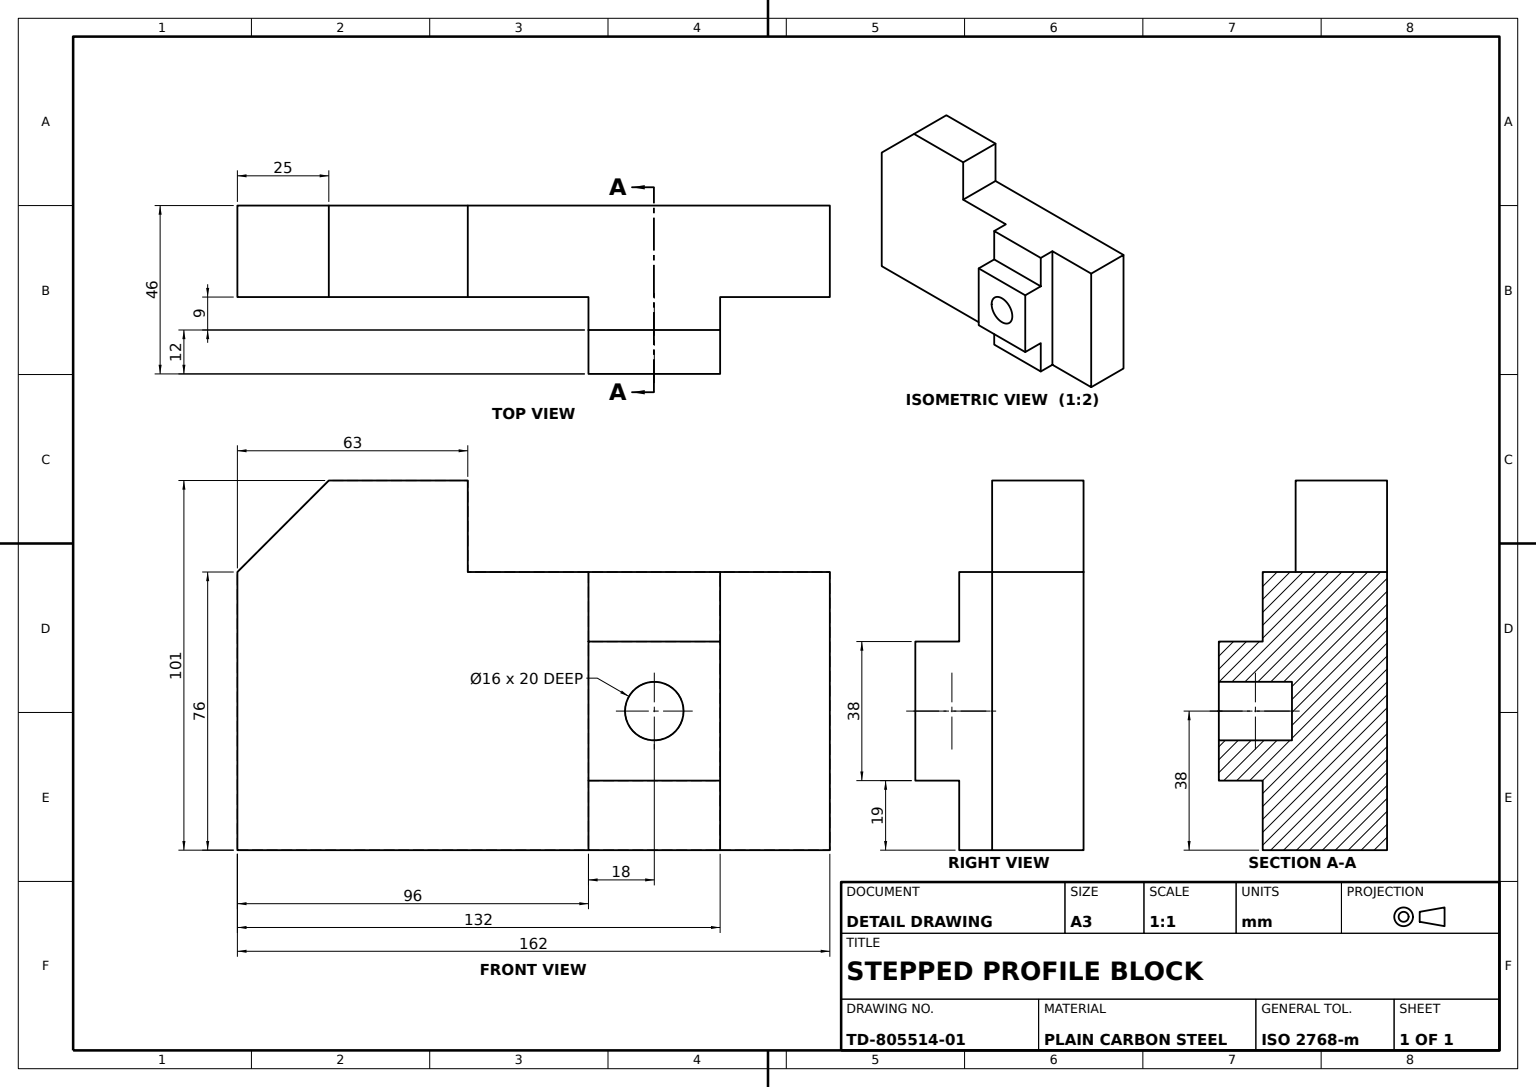
from build123d import *

# Parameters (mm, degrees)
BASE_BLOCK_DEPTH   = 25
SIDE_BLOCK_DEPTH   = 25
PAD_SKETCH_W       = 36
PAD_SKETCH_H       = 76
MOUNTING_PAD_DEPTH = 9
LUG_BOSS_SKETCH_W  = 36
LUG_BOSS_SKETCH_H  = 38
LUG_BOSS_DEPTH     = 12
HOLE_SKETCH_16_R   = 8
HOLE_16_DEPTH      = 20


with BuildPart() as part:
    # Base Profile Sketch → Base Block (new body)
    with BuildSketch(Plane.XY):
        Polygon((0, 0), (162, 0), (162, 76), (25, 76), (0, 76), (0, 51), align=None)
    extrude(amount=BASE_BLOCK_DEPTH)

    # Side Block Sketch → Side Block (add)
    with BuildSketch(Plane.XY.offset(25)):
        Polygon((63, 76), (63, 101), (25, 101), (0, 76), (25, 76), align=None)
    extrude(amount=-SIDE_BLOCK_DEPTH)

    # Pad Sketch → Mounting Pad (add)
    with BuildSketch(Plane.XY.offset(25)):
        with Locations((114, 38)):
            Rectangle(PAD_SKETCH_W, PAD_SKETCH_H)
    extrude(amount=MOUNTING_PAD_DEPTH)

    # Lug Boss Sketch → Lug Boss (add)
    with BuildSketch(Plane.XY.offset(34)):
        with Locations((114, 38)):
            Rectangle(LUG_BOSS_SKETCH_W, LUG_BOSS_SKETCH_H)
    extrude(amount=LUG_BOSS_DEPTH)

    # Hole Sketch Ø16 → Hole Ø16 (cut)
    with BuildSketch(Plane.XY.offset(46)):
        with Locations((114, 38)):
            Circle(HOLE_SKETCH_16_R)
    extrude(amount=-HOLE_16_DEPTH, mode=Mode.SUBTRACT)


solid = part.part
